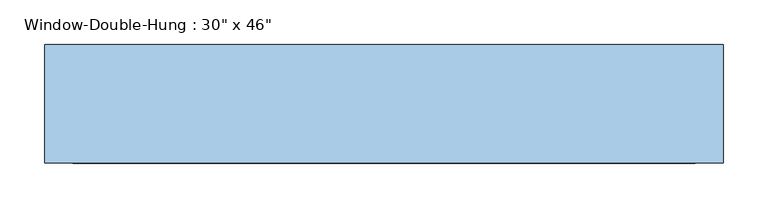
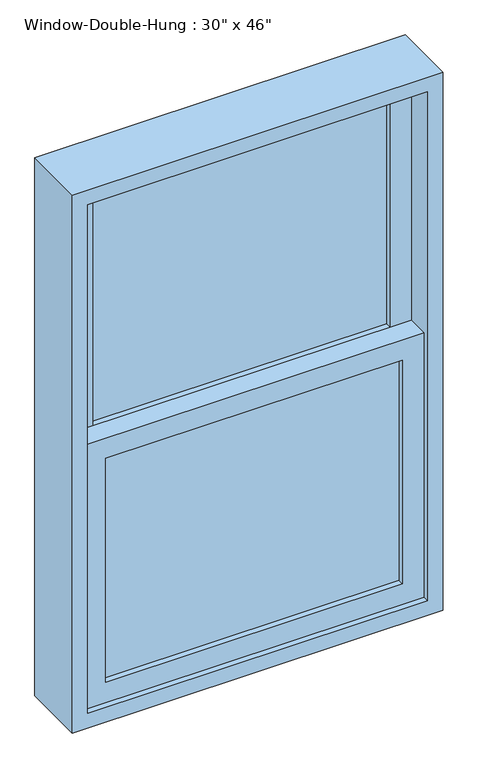
"""IFC4 building model written with IfcOpenShell, lengths in millimetres: window geometry."""

from ifc_helpers import new_model, si_unit, frame, origin, place, context, project, spatial, polyline, outline, extrude, source, transform, mapped, element, save


def window_5a369d27(model_context):
    return source(origin(), model_context, "Body", "SweptSolid", [
        extrude(outline(polyline([(304.8, -12.7), (304.8, -19.05), (-304.8, -19.05), (-304.8, -12.7), (304.8, -12.7)])), frame((0.0, 0.0, 990.6), z_axis=(0.0, 0.0, 1.0), x_axis=(1.0, 0.0, 0.0)), (0.0, 0.0, 1.0), 485.775),
        extrude(outline(polyline([(-304.8, -25.4), (304.8, -25.4), (304.8, -31.75), (-304.8, -31.75), (-304.8, -25.4)])), frame((0.0, 0.0, 990.6), z_axis=(0.0, 0.0, 1.0), x_axis=(1.0, 0.0, 0.0)), (0.0, 0.0, 1.0), 485.775),
        extrude(outline(polyline([(304.8, 31.75), (304.8, 25.4), (-304.8, 25.4), (-304.8, 31.75), (304.8, 31.75)])), frame((0.0, 0.0, 1520.825), z_axis=(0.0, 0.0, 1.0), x_axis=(1.0, 0.0, 0.0)), (0.0, 0.0, 1.0), 485.775),
        extrude(outline(polyline([(-304.8, 19.05), (304.8, 19.05), (304.8, 12.7), (-304.8, 12.7), (-304.8, 19.05)])), frame((0.0, 0.0, 1520.825), z_axis=(0.0, 0.0, 1.0), x_axis=(1.0, 0.0, 0.0)), (0.0, 0.0, 1.0), 485.775),
        extrude(outline(polyline([(1520.825, -349.25), (946.15, -349.25), (946.15, 349.25), (1520.825, 349.25), (1520.825, -349.25)]), holes=[polyline([(1476.375, 304.8), (990.6, 304.8), (990.6, -304.8), (1476.375, -304.8), (1476.375, 304.8)])]), frame((0.0, -44.45, 0.0), z_axis=(0.0, 1.0, 0.0), x_axis=(0.0, 0.0, 1.0)), (0.0, 0.0, 1.0), 44.45),
        extrude(outline(polyline([(2051.05, -349.25), (1476.375, -349.25), (1476.375, 349.25), (2051.05, 349.25), (2051.05, -349.25)]), holes=[polyline([(2006.6, 304.8), (1520.825, 304.8), (1520.825, -304.8), (2006.6, -304.8), (2006.6, 304.8)])]), frame((0.0, 0.0, 0.0), z_axis=(0.0, 1.0, 0.0), x_axis=(0.0, 0.0, 1.0)), (0.0, 0.0, 1.0), 44.45),
        extrude(outline(polyline([(2082.8, -381.0), (914.4, -381.0), (914.4, 381.0), (2082.8, 381.0), (2082.8, -381.0)]), holes=[polyline([(2051.05, 349.25), (946.15, 349.25), (946.15, -349.25), (2051.05, -349.25), (2051.05, 349.25)])]), frame((0.0, -57.15, 0.0), z_axis=(0.0, 1.0, 0.0), x_axis=(0.0, 0.0, 1.0)), (0.0, 0.0, 1.0), 133.35),
    ])


if __name__ == "__main__":
    model = new_model("IFC4")
    model_context = context("Model", 3, world=origin())
    ifc_project = project(units=[si_unit("LENGTHUNIT", "METRE", prefix="MILLI")], contexts=[model_context])
    site = spatial("IfcSite", under=ifc_project)
    building = spatial("IfcBuilding", under=site)
    placement = place(None, origin())
    window_shape = window_5a369d27(model_context)
    element("IfcWindow", 1, ObjectType="Window-Double-Hung : 30\" x 46\"", at=placement, inside=building, context=model_context, shape_type="MappedRepresentation", body=[
        mapped(window_shape, transform((0.0, 0.0, 0.0), x_axis=(1.0, 0.0, 0.0), y_axis=(0.0, 1.0, 0.0), z_axis=(0.0, 0.0, 1.0))),
    ])
    save(model, "model.ifc")

# Revit data of these elements
# Type "Window-Double-Hung : 30\" x 46\""
#   Type Mark = "13"
#   Fire Rating = "0.5h"
#   Construction Type Id = "DG-DR"
#   Assembly Code = "B2020100"
#   Analytic Construction = "Double glazing - domestic"
#   Wall Thickness [instance default] = 0' - 6"
#   Window Inset [instance default] = 0' - 0"
#   Visual Light Transmittance = 0.81
#   Thermal Resistance (R) = 1.8146 (h·ft²·°F)/BTU
#   Solar Heat Gain Coefficient = 0.76
#   Muntin Width = 2' - 0"
#   Muntin Height = 1' - 7 1/8"
#   Interior Wall Closure [instance default] = 0' - 1 1/2"
#   Rough Width = 2' - 6 1/2"
#   Rough Height = 3' - 10 1/2"
#   Frame Extension [instance default] = 0' - 1 1/4"
#   Exterior Wall Closure [instance default] = 0' - 0 1/2"
#   Extension Jamb [instance default] = 0' - 1 1/2"
#   Heat Transfer Coefficient (U) = 0.5511 BTU/(h·ft²·°F)
#   Height = 3' - 10"
#   Width = 2' - 6"
#   Define Thermal Properties by = 1
#   Top Muntin Visibility = yes
#   Indicator Visibility [instance default] = yes
#   Extension Jamb Visibility [instance default] = yes
#   Interior Trim Visibility [instance default] = yes
#   Exterior Trim Visibility [instance default] = yes
#   Define Thermal Properties by = 1
#   Bottom Muntin Visibility = yes
#   Muntin Pattern = Muntin Pattern_2x2 : Muntin Pattern_2x2
#   Interior Trim Material = Wood - Stained
#   Interior Trim = Trim-Window-Interior-Flat : Picture Frame
#   Exterior Trim Material = Clad - White
#   Exterior Trim = Trim-Window-Exterior-Flat : with Sill
#   Glass Panel Material = Glass
#   Exterior Frame Material = Clad - White
#   Interior Frame Material = Wood - Stained
#   Wall Closure = (empty or 0)
# Element 1 (IfcWindow, "Window-Double-Hung : 30\" x 46\"")
#   Wall Thickness = 0' - 4 1/2"
#   Extension Jamb = 0' - 1"
#   Extension Jamb Visibility = no
#   Materials on its faces: "Wood - Stained", "Glass", "Clad - White"
# Materials
#   "Wood - Stained": class "Wood", colour RGB 224 178 126, transparency 0, Cost = 0
#   "Clad - White": class "Wood", colour RGB 242 242 238, transparency 0, Cost = 0
#   "Glass": class "Glass", colour RGB 0 128 192, transparency 0.75, Description = "Soda Lime Glass", Cost = 0
